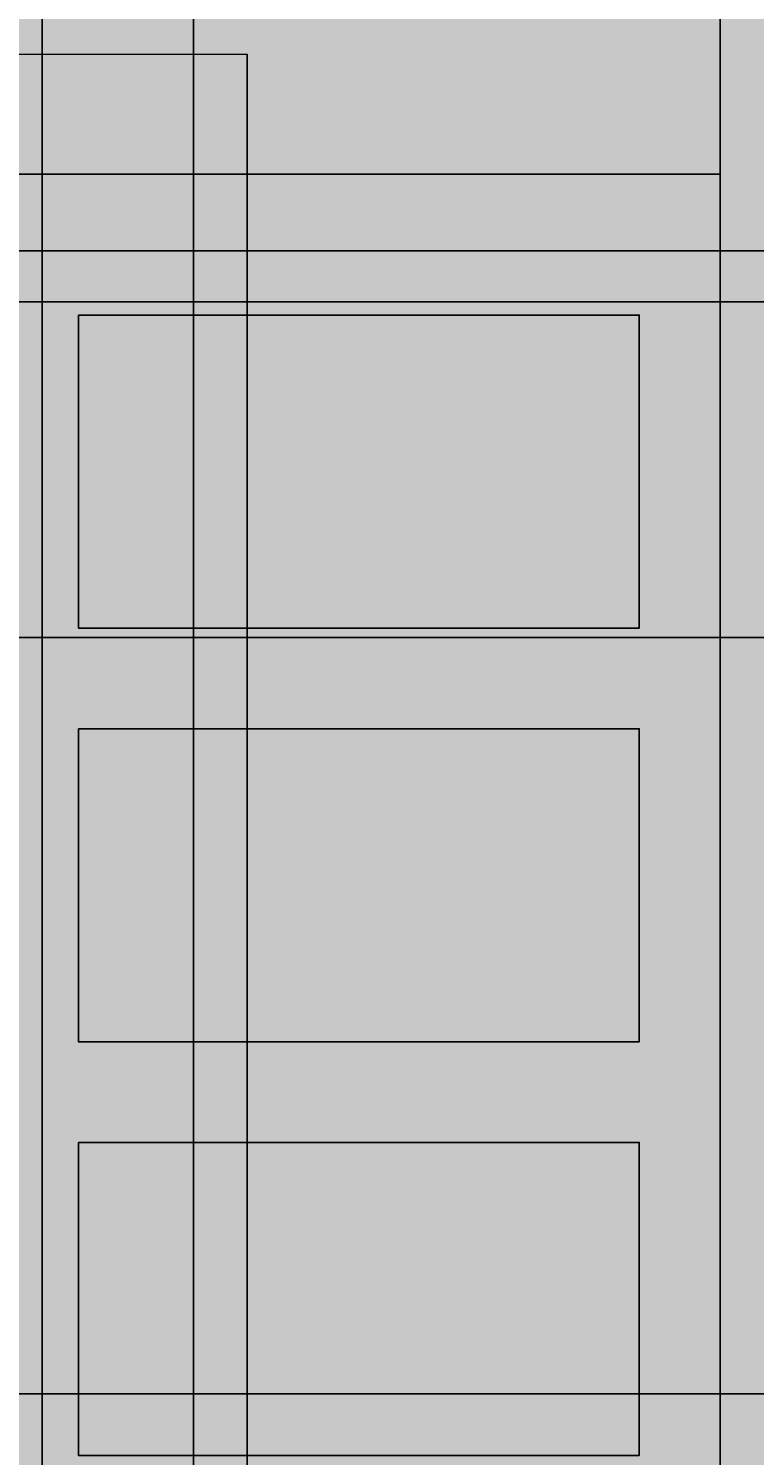
# Model space of a CAD drawing. Units: inches. Extents: x 3024 to 4744, y 1110 to 2100.
# Tile 7 of 29: x 3275 to 3332, y 1181 to 1293. Entities that reach past the tile are written whole.
import ezdxf

# ---------------------------------------------------------------- set-up
doc = ezdxf.new("R2010")
doc.units = ezdxf.units.IN
for name, color, linetype, lineweight in [('A-ANNO-DIMS', 2, 'Continuous', 18), ('A-ELEV', 7, 'Continuous', 25), ('A-ELEV-PATT', 252, 'Continuous', 13), ('A-GLAZ', 4, 'Continuous', 18)]:
    doc.layers.add(name, color=color, linetype=linetype, lineweight=lineweight)
doc.styles.get("Standard").update_dxf_attribs({"font": 'arial.ttf'})
doc.dimstyles.get("Standard").update_dxf_attribs({"dimtxt": 0.18, "dimasz": 0.18, "dimexe": 0.18, "dimexo": 0.0625, "dimgap": 0.09, "dimtad": 0, "dimtih": 1, "dimtoh": 1, "dimdec": 1, "dimzin": 0, "dimdsep": 46, "dimlunit": 3, "dimtxsty": 'Standard', "dimcen": 0.09, "dimadec": 0, "dimazin": 0, "dimtfac": 1, "dimtdec": 1, "dimtofl": 0, "dimtmove": 0, "dimatfit": 3, "dimfxl": 1, "dimtolj": 1, "dimtzin": 0, "dimarcsym": 0})

# ---------------------------------------------------------------- blocks, each defined once
blk = doc.blocks.new('WIN-BALCONY-A')
blk.add_line((3169.4, 1795.04), (3292.61, 1795.04))
blk.add_line((3169.4, 1795.04), (3292.61, 1795.04))
blk.add_lwpolyline([(3276.51, 1795.04), (3288.38, 1795.04), (3288.38, 1806.87), (3276.51, 1806.87)], close=True)
blk.add_lwpolyline([(3276.51, 1795.04), (3288.38, 1795.04), (3288.38, 1806.87), (3276.51, 1806.87)], close=True)
blk.add_lwpolyline([(3292.61, 1795.04), (3292.61, 1785.61), (3148.97, 1785.61), (3148.97, 1795.04)])
blk.add_lwpolyline([(3292.61, 1795.04), (3292.61, 1785.61), (3148.97, 1785.61), (3148.97, 1795.04)])
blk = doc.blocks.new('*D54')
at = {"layer": 'A-ANNO-DIMS', "color": 0, "lineweight": -2, "transparency": 16777216}
for p, q in [((3292.61, 1290.98), (3292.61, 1109.93)), ((3274.39, 1170.96), (3274.39, 1109.93)), ((3274.57, 1110.11), (3283.04, 1110.11)), ((3292.43, 1110.11), (3283.95, 1110.11))]:
    blk.add_line(p, q, dxfattribs=at)
at = {"layer": 'A-ANNO-DIMS', "color": 0, "transparency": 16777216}
for points in [[(3274.57, 1110.14), (3274.57, 1110.08), (3274.39, 1110.11)], [(3292.43, 1110.14), (3292.43, 1110.08), (3292.61, 1110.11)]]:
    blk.add_solid(points, dxfattribs=at)
at = {"layer": 'Defpoints', "color": 0, "transparency": 16777216}
for p in [(3292.61, 1291.04), (3274.39, 1171.02), (3292.61, 1110.11)]:
    blk.add_point(p, dxfattribs=at)
at = {"layer": 'A-ANNO-DIMS', "color": 0, "transparency": 16777216, "insert": (3283.5, 1110.11), "char_height": 0.18, "attachment_point": 5}
blk.add_mtext('\\A1;18.217', dxfattribs=at)
blk = doc.blocks.new('*D55')
at = {"layer": 'A-ANNO-DIMS', "color": 0, "lineweight": -2, "transparency": 16777216}
for p, q in [((3292.61, 1290.98), (3292.61, 1109.93)), ((3329.7, 1155.55), (3329.7, 1109.93)), ((3292.79, 1110.11), (3310.85, 1110.11)), ((3329.52, 1110.11), (3311.46, 1110.11))]:
    blk.add_line(p, q, dxfattribs=at)
at = {"layer": 'A-ANNO-DIMS', "color": 0, "transparency": 16777216}
for points in [[(3292.79, 1110.14), (3292.79, 1110.08), (3292.61, 1110.11)], [(3329.52, 1110.14), (3329.52, 1110.08), (3329.7, 1110.11)]]:
    blk.add_solid(points, dxfattribs=at)
at = {"layer": 'Defpoints', "color": 0, "transparency": 16777216}
for p in [(3292.61, 1291.04), (3329.7, 1155.61), (3329.7, 1110.11)]:
    blk.add_point(p, dxfattribs=at)
at = {"layer": 'A-ANNO-DIMS', "color": 0, "transparency": 16777216, "insert": (3311.15, 1110.11), "char_height": 0.18, "attachment_point": 5}
blk.add_mtext('\\A1;37.1', dxfattribs=at)
blk = doc.blocks.new('*D56')
at = {"layer": 'A-ANNO-DIMS', "color": 0, "lineweight": -2, "transparency": 16777216}
for p, q in [((3361.22, 1329.46), (3361.22, 1109.93)), ((3329.7, 1155.55), (3329.7, 1109.93)), ((3329.88, 1110.11), (3345.07, 1110.11)), ((3361.04, 1110.11), (3345.86, 1110.11))]:
    blk.add_line(p, q, dxfattribs=at)
at = {"layer": 'A-ANNO-DIMS', "color": 0, "transparency": 16777216}
for points in [[(3329.88, 1110.14), (3329.88, 1110.08), (3329.7, 1110.11)], [(3361.04, 1110.14), (3361.04, 1110.08), (3361.22, 1110.11)]]:
    blk.add_solid(points, dxfattribs=at)
at = {"layer": 'Defpoints', "color": 0, "transparency": 16777216}
for p in [(3361.22, 1329.52), (3329.7, 1155.61), (3361.22, 1110.11)]:
    blk.add_point(p, dxfattribs=at)
at = {"layer": 'A-ANNO-DIMS', "color": 0, "transparency": 16777216, "insert": (3345.46, 1110.11), "char_height": 0.18, "attachment_point": 5}
blk.add_mtext('\\A1;31.52', dxfattribs=at)
blk = doc.blocks.new('*D64')
at = {"layer": 'A-ANNO-DIMS', "color": 0, "lineweight": -2, "transparency": 16777216}
for p, q in [((3069.79, 1241.5), (3069.79, 2100.44)), ((3069.97, 2100.26), (3405.08, 2100.26)), ((3740.97, 2100.26), (3405.87, 2100.26)), ((3741.15, 1241.5), (3741.15, 2100.44))]:
    blk.add_line(p, q, dxfattribs=at)
at = {"layer": 'A-ANNO-DIMS', "color": 0, "transparency": 16777216}
for points in [[(3069.97, 2100.29), (3069.97, 2100.23), (3069.79, 2100.26)], [(3740.97, 2100.29), (3740.97, 2100.23), (3741.15, 2100.26)]]:
    blk.add_solid(points, dxfattribs=at)
at = {"layer": 'Defpoints', "color": 0, "transparency": 16777216}
for p in [(3741.15, 2100.26), (3069.79, 1241.43), (3741.15, 1241.43)]:
    blk.add_point(p, dxfattribs=at)
at = {"layer": 'A-ANNO-DIMS', "color": 0, "transparency": 16777216, "insert": (3405.47, 2100.26), "char_height": 0.18, "attachment_point": 5}
blk.add_mtext('\\A1;671.4', dxfattribs=at)
blk = doc.blocks.new('*D94')
at = {"layer": 'A-ANNO-DIMS', "color": 0, "lineweight": -2, "transparency": 16777216}
for p, q in [((3276.51, 1794.98), (3276.51, 1109.93)), ((3288.38, 1794.98), (3288.38, 1109.93)), ((3276.69, 1110.11), (3281.99, 1110.11)), ((3288.2, 1110.11), (3282.9, 1110.11))]:
    blk.add_line(p, q, dxfattribs=at)
at = {"layer": 'A-ANNO-DIMS', "color": 0, "transparency": 16777216}
for points in [[(3276.69, 1110.14), (3276.69, 1110.08), (3276.51, 1110.11)], [(3288.2, 1110.14), (3288.2, 1110.08), (3288.38, 1110.11)]]:
    blk.add_solid(points, dxfattribs=at)
at = {"layer": 'Defpoints', "color": 0, "transparency": 16777216}
for p in [(3276.51, 1795.04), (3288.38, 1795.04), (3288.38, 1110.11)]:
    blk.add_point(p, dxfattribs=at)
at = {"layer": 'A-ANNO-DIMS', "color": 0, "transparency": 16777216, "insert": (3282.44, 1110.11), "char_height": 0.18, "attachment_point": 5}
blk.add_mtext('\\A1;11.866', dxfattribs=at)
blk = doc.blocks.new('*D120')
at = {"layer": 'A-ANNO-DIMS', "color": 0, "lineweight": -2, "transparency": 16777216}
for p, q in [((3270.45, 1271.61), (3786.83, 1271.61)), ((3786.65, 1271.43), (3786.65, 1221.5)), ((3786.65, 1171.2), (3786.65, 1221.14)), ((3274.45, 1171.02), (3786.83, 1171.02))]:
    blk.add_line(p, q, dxfattribs=at)
at = {"layer": 'A-ANNO-DIMS', "color": 0, "transparency": 16777216}
for points in [[(3786.62, 1271.43), (3786.68, 1271.43), (3786.65, 1271.61)], [(3786.62, 1171.2), (3786.68, 1171.2), (3786.65, 1171.02)]]:
    blk.add_solid(points, dxfattribs=at)
at = {"layer": 'Defpoints', "color": 0, "transparency": 16777216}
for p in [(3270.39, 1271.61), (3786.65, 1271.61), (3274.39, 1171.02)]:
    blk.add_point(p, dxfattribs=at)
at = {"layer": 'A-ANNO-DIMS', "color": 0, "transparency": 16777216, "insert": (3786.65, 1221.32), "char_height": 0.18, "attachment_point": 5}
blk.add_mtext('\\A1;100.59', dxfattribs=at)
blk = doc.blocks.new('*D121')
at = {"layer": 'A-ANNO-DIMS', "color": 0, "lineweight": -2, "transparency": 16777216}
for p, q in [((3274.45, 1275.61), (3786.83, 1275.61)), ((3786.65, 1275.43), (3786.65, 1273.79)), ((3786.65, 1271.79), (3786.65, 1273.43)), ((3270.45, 1271.61), (3786.83, 1271.61))]:
    blk.add_line(p, q, dxfattribs=at)
at = {"layer": 'A-ANNO-DIMS', "color": 0, "transparency": 16777216}
for points in [[(3786.62, 1275.43), (3786.68, 1275.43), (3786.65, 1275.61)], [(3786.62, 1271.79), (3786.68, 1271.79), (3786.65, 1271.61)]]:
    blk.add_solid(points, dxfattribs=at)
at = {"layer": 'Defpoints', "color": 0, "transparency": 16777216}
for p in [(3274.39, 1275.61), (3786.65, 1275.61), (3270.39, 1271.61)]:
    blk.add_point(p, dxfattribs=at)
at = {"layer": 'A-ANNO-DIMS', "color": 0, "transparency": 16777216, "insert": (3786.65, 1273.61), "char_height": 0.18, "attachment_point": 5}
blk.add_mtext('\\A1;4.00', dxfattribs=at)
blk = doc.blocks.new('*D122')
at = {"layer": 'A-ANNO-DIMS', "color": 0, "lineweight": -2, "transparency": 16777216}
for p, q in [((3228.45, 1185.95), (3786.83, 1185.95)), ((3786.65, 1185.77), (3786.65, 1178.67)), ((3786.65, 1171.2), (3786.65, 1178.31)), ((3270.45, 1171.02), (3786.83, 1171.02))]:
    blk.add_line(p, q, dxfattribs=at)
at = {"layer": 'A-ANNO-DIMS', "color": 0, "transparency": 16777216}
for points in [[(3786.62, 1185.77), (3786.68, 1185.77), (3786.65, 1185.95)], [(3786.62, 1171.2), (3786.68, 1171.2), (3786.65, 1171.02)]]:
    blk.add_solid(points, dxfattribs=at)
at = {"layer": 'Defpoints', "color": 0, "transparency": 16777216}
for p in [(3228.39, 1185.95), (3270.39, 1171.02), (3786.65, 1171.02)]:
    blk.add_point(p, dxfattribs=at)
at = {"layer": 'A-ANNO-DIMS', "color": 0, "transparency": 16777216, "insert": (3786.65, 1178.49), "char_height": 0.18, "attachment_point": 5}
blk.add_mtext('\\A1;14.928', dxfattribs=at)
blk = doc.blocks.new('*D123')
at = {"layer": 'A-ANNO-DIMS', "color": 0, "lineweight": -2, "transparency": 16777216}
for p, q in [((3228.45, 1245.27), (3786.83, 1245.27)), ((3786.65, 1245.09), (3786.65, 1215.79)), ((3786.65, 1186.13), (3786.65, 1215.43)), ((3228.45, 1185.95), (3786.83, 1185.95))]:
    blk.add_line(p, q, dxfattribs=at)
at = {"layer": 'A-ANNO-DIMS', "color": 0, "transparency": 16777216}
for points in [[(3786.62, 1245.09), (3786.68, 1245.09), (3786.65, 1245.27)], [(3786.62, 1186.13), (3786.68, 1186.13), (3786.65, 1185.95)]]:
    blk.add_solid(points, dxfattribs=at)
at = {"layer": 'Defpoints', "color": 0, "transparency": 16777216}
for p in [(3228.39, 1245.27), (3786.65, 1245.27), (3228.39, 1185.95)]:
    blk.add_point(p, dxfattribs=at)
at = {"layer": 'A-ANNO-DIMS', "color": 0, "transparency": 16777216, "insert": (3786.65, 1215.61), "char_height": 0.18, "attachment_point": 5}
blk.add_mtext('\\A1;59.32', dxfattribs=at)

msp = doc.modelspace()

# ---------------------------------------------------------------- hatches: boundary and pattern name
at = {"layer": 'A-ELEV-PATT'}
h = msp.add_hatch(color=256, dxfattribs=at)
h.dxf.hatch_style = 1
h.paths.add_polyline_path([(3491.8271, 2054.7584), (3320.5658, 2054.7584), (3320.5658, 2043.5286), (3491.8271, 2043.5286)])
h.paths.add_polyline_path([(3292.6051, 1905.6112), (3148.9694, 1905.6112), (3148.9694, 1897.4879), (3169.3964, 1897.4879), (3292.6051, 1897.4879)])
h.paths.add_polyline_path([(3292.6051, 1795.0431), (3169.3964, 1795.0431), (3148.9694, 1795.0431), (3148.9694, 1785.6112), (3292.6051, 1785.6112)])
h.paths.add_polyline_path([(3292.6051, 1779.6112), (3148.9694, 1779.6112), (3148.9694, 1771.4879), (3169.3964, 1771.4879), (3292.6051, 1771.4879)])
h.paths.add_polyline_path([(3292.6051, 1669.0431), (3169.3964, 1669.0431), (3148.9694, 1669.0431), (3148.9694, 1659.6112), (3292.6051, 1659.6112)])
h.paths.add_polyline_path([(3292.6051, 1653.6112), (3148.9694, 1653.6112), (3148.9694, 1645.4879), (3169.3964, 1645.4879), (3292.6051, 1645.4879)])
h.paths.add_polyline_path([(3292.6051, 1543.0431), (3169.3964, 1543.0431), (3148.9694, 1543.0431), (3148.9694, 1533.6112), (3292.6051, 1533.6112)])
h.paths.add_polyline_path([(3292.6051, 1527.6112), (3148.9694, 1527.6112), (3148.9694, 1519.4879), (3169.3964, 1519.4879), (3292.6051, 1519.4879)])
h.paths.add_polyline_path([(3292.6051, 1401.6112), (3148.9694, 1401.6112), (3148.9694, 1393.4879), (3169.3964, 1393.4879), (3292.6051, 1393.4879)])
h.paths.add_polyline_path([(3292.6051, 1417.0431), (3169.3964, 1417.0431), (3148.9694, 1417.0431), (3148.9694, 1407.6112), (3292.6051, 1407.6112)])
h.paths.add_polyline_path([(3292.6051, 1291.0431), (3169.3964, 1291.0431), (3148.9694, 1291.0431), (3148.9694, 1281.6112), (3292.6051, 1281.6112)])
h.paths.add_polyline_path([(3654.037, 1165.0431), (3530.8283, 1165.0431), (3510.4013, 1165.0431), (3510.4013, 1155.6112), (3654.037, 1155.6112)])
h.paths.add_polyline_path([(3654.037, 1275.6112), (3510.4013, 1275.6112), (3510.4013, 1267.4879), (3530.8283, 1267.4879), (3654.037, 1267.4879)])
h.paths.add_polyline_path([(3654.037, 1291.0431), (3530.8283, 1291.0431), (3510.4013, 1291.0431), (3510.4013, 1281.6112), (3654.037, 1281.6112)])
h.paths.add_polyline_path([(3654.037, 1417.0431), (3530.8283, 1417.0431), (3510.4013, 1417.0431), (3510.4013, 1407.6112), (3654.037, 1407.6112)])
h.paths.add_polyline_path([(3654.037, 1401.6112), (3510.4013, 1401.6112), (3510.4013, 1393.4879), (3530.8283, 1393.4879), (3654.037, 1393.4879)])
h.paths.add_polyline_path([(3654.037, 1543.0431), (3530.8283, 1543.0431), (3510.4013, 1543.0431), (3510.4013, 1533.6112), (3654.037, 1533.6112)])
h.paths.add_polyline_path([(3654.037, 1527.6112), (3510.4013, 1527.6112), (3510.4013, 1519.4879), (3530.8283, 1519.4879), (3654.037, 1519.4879)])
h.paths.add_polyline_path([(3654.037, 1653.6112), (3510.4013, 1653.6112), (3510.4013, 1645.4879), (3530.8283, 1645.4879), (3654.037, 1645.4879)])
h.paths.add_polyline_path([(3654.037, 1669.0431), (3530.8283, 1669.0431), (3510.4013, 1669.0431), (3510.4013, 1659.6112), (3654.037, 1659.6112)])
h.paths.add_polyline_path([(3654.037, 1779.6112), (3510.4013, 1779.6112), (3510.4013, 1771.4879), (3530.8283, 1771.4879), (3654.037, 1771.4879)])
h.paths.add_polyline_path([(3654.037, 1795.0431), (3530.8283, 1795.0431), (3510.4013, 1795.0431), (3510.4013, 1785.6112), (3654.037, 1785.6112)])
h.paths.add_polyline_path([(3654.037, 1905.6112), (3510.4013, 1905.6112), (3510.4013, 1897.4879), (3530.8283, 1897.4879), (3654.037, 1897.4879)])
h = msp.add_hatch(color=256, dxfattribs=at)
h.dxf.hatch_style = 1
h.paths.add_polyline_path([(3335.1044, 2043.5286), (3329.7033, 2043.5286), (3329.7033, 1155.6112), (3335.1044, 1155.6112)])
h.paths.add_polyline_path([(3481.2411, 2043.5286), (3335.1044, 2043.5286), (3335.1044, 1155.6112), (3481.2411, 1155.6112)])
h.paths.add_polyline_path([(3449.7202, 1329.5246), (3361.2242, 1329.5246), (3361.2242, 1436.6064), (3449.7202, 1436.6064)], flags=16)
h.paths.add_polyline_path([(3445.7202, 1333.5246), (3365.2242, 1333.5246), (3365.2242, 1432.6064), (3445.7202, 1432.6064)], flags=0)
h.paths.add_polyline_path([(3449.7202, 1455.5246), (3361.2242, 1455.5246), (3361.2242, 1562.6064), (3449.7202, 1562.6064)], flags=16)
h.paths.add_polyline_path([(3445.7202, 1459.5246), (3365.2242, 1459.5246), (3365.2242, 1558.6064), (3445.7202, 1558.6064)], flags=0)
h.paths.add_polyline_path([(3449.7202, 1581.5246), (3361.2242, 1581.5246), (3361.2242, 1688.6064), (3449.7202, 1688.6064)], flags=16)
h.paths.add_polyline_path([(3445.7202, 1585.5246), (3365.2242, 1585.5246), (3365.2242, 1684.6064), (3445.7202, 1684.6064)], flags=0)
h.paths.add_polyline_path([(3449.7202, 1707.5246), (3361.2242, 1707.5246), (3361.2242, 1814.6064), (3449.7202, 1814.6064)], flags=16)
h.paths.add_polyline_path([(3445.7202, 1711.5246), (3365.2242, 1711.5246), (3365.2242, 1810.6064), (3445.7202, 1810.6064)], flags=0)
h.paths.add_polyline_path([(3449.7202, 1833.5246), (3361.2242, 1833.5246), (3361.2242, 1940.6064), (3449.7202, 1940.6064)], flags=16)
h.paths.add_polyline_path([(3445.7202, 1837.5246), (3365.2242, 1837.5246), (3365.2242, 1936.6064), (3445.7202, 1936.6064)], flags=0)
h = msp.add_hatch(color=256, dxfattribs=at)
h.dxf.hatch_style = 1
h.paths.add_polyline_path([(3329.7033, 1407.6112), (3105.4722, 1407.6112), (3105.4722, 1401.6112), (3329.7033, 1401.6112)])
h.paths.add_polyline_path([(3329.7033, 1281.6112), (3105.4722, 1281.6112), (3105.4722, 1275.6112), (3112.3838, 1275.6112), (3329.7033, 1275.6112)])
h.paths.add_polyline_path([(3329.7033, 1533.6112), (3105.4722, 1533.6112), (3105.4722, 1527.6112), (3329.7033, 1527.6112)])
h.paths.add_polyline_path([(3329.7033, 1659.6112), (3105.4722, 1659.6112), (3105.4722, 1653.6112), (3329.7033, 1653.6112)])
h.paths.add_polyline_path([(3329.7033, 1785.6112), (3105.4722, 1785.6112), (3105.4722, 1779.6112), (3329.7033, 1779.6112)])
h.paths.add_polyline_path([(3329.7033, 1911.6112), (3105.4722, 1911.6112), (3095.7158, 1911.6112), (3095.7158, 1905.6112), (3329.7033, 1905.6112)])
h.paths.add_polyline_path([(3715.2286, 1911.6112), (3705.4722, 1911.6112), (3705.4722, 1905.6112), (3715.2286, 1905.6112)])
h.paths.add_polyline_path([(3688.5588, 1911.6112), (3481.2411, 1911.6112), (3481.2411, 1905.6112), (3688.5588, 1905.6112)])
h = msp.add_hatch(color=256, dxfattribs=at)
h.dxf.hatch_style = 1
h.paths.add_polyline_path([(3154.3287, 1897.4879), (3148.9694, 1897.4879), (3148.9694, 1905.6112), (3105.4722, 1905.6112), (3105.4722, 1785.6112), (3148.9694, 1785.6112), (3148.9694, 1795.0431), (3151.6604, 1795.0431), (3151.6604, 1806.8674), (3154.3287, 1806.8674)])
h.paths.add_polyline_path([(3329.7033, 1905.6112), (3292.6051, 1905.6112), (3292.6051, 1897.4879), (3287.2458, 1897.4879), (3287.2458, 1806.8674), (3288.3759, 1806.8674), (3288.3759, 1795.0431), (3292.6051, 1795.0431), (3292.6051, 1785.6112), (3329.7033, 1785.6112)])
h.paths.add_polyline_path([(3154.3287, 1771.4879), (3148.9694, 1771.4879), (3148.9694, 1779.6112), (3105.4722, 1779.6112), (3105.4722, 1659.6112), (3148.9694, 1659.6112), (3148.9694, 1669.0431), (3151.6604, 1669.0431), (3151.6604, 1680.8674), (3154.3287, 1680.8674)])
h.paths.add_polyline_path([(3329.7033, 1779.6112), (3292.6051, 1779.6112), (3292.6051, 1771.4879), (3287.2458, 1771.4879), (3287.2458, 1680.8674), (3288.3759, 1680.8674), (3288.3759, 1669.0431), (3292.6051, 1669.0431), (3292.6051, 1659.6112), (3329.7033, 1659.6112)])
h.paths.add_polyline_path([(3154.3287, 1645.4879), (3148.9694, 1645.4879), (3148.9694, 1653.6112), (3105.4722, 1653.6112), (3105.4722, 1533.6112), (3148.9694, 1533.6112), (3148.9694, 1543.0431), (3151.6604, 1543.0431), (3151.6604, 1554.8674), (3154.3287, 1554.8674)])
h.paths.add_polyline_path([(3329.7033, 1653.6112), (3292.6051, 1653.6112), (3292.6051, 1645.4879), (3287.2458, 1645.4879), (3287.2458, 1554.8674), (3288.3759, 1554.8674), (3288.3759, 1543.0431), (3292.6051, 1543.0431), (3292.6051, 1533.6112), (3329.7033, 1533.6112)])
h.paths.add_polyline_path([(3329.7033, 1527.6112), (3292.6051, 1527.6112), (3292.6051, 1519.4879), (3287.2458, 1519.4879), (3287.2458, 1428.8674), (3288.3759, 1428.8674), (3288.3759, 1417.0431), (3292.6051, 1417.0431), (3292.6051, 1407.6112), (3329.7033, 1407.6112)])
h.paths.add_polyline_path([(3329.7033, 1401.6112), (3292.6051, 1401.6112), (3292.6051, 1393.4879), (3287.2458, 1393.4879), (3287.2458, 1302.8674), (3288.3759, 1302.8674), (3288.3759, 1291.0431), (3292.6051, 1291.0431), (3292.6051, 1281.6112), (3329.7033, 1281.6112)])
h.paths.add_polyline_path([(3154.3287, 1393.4879), (3148.9694, 1393.4879), (3148.9694, 1401.6112), (3105.4722, 1401.6112), (3105.4722, 1281.6112), (3148.9694, 1281.6112), (3148.9694, 1291.0431), (3151.6604, 1291.0431), (3151.6604, 1302.8674), (3154.3287, 1302.8674)])
h.paths.add_polyline_path([(3154.3287, 1519.4879), (3148.9694, 1519.4879), (3148.9694, 1527.6112), (3105.4722, 1527.6112), (3105.4722, 1407.6112), (3148.9694, 1407.6112), (3148.9694, 1417.0431), (3151.6604, 1417.0431), (3151.6604, 1428.8674), (3154.3287, 1428.8674)])
h.paths.add_polyline_path([(3515.7606, 1897.4879), (3510.4013, 1897.4879), (3510.4013, 1905.6112), (3481.2411, 1905.6112), (3481.2411, 1785.6112), (3510.4013, 1785.6112), (3510.4013, 1795.0431), (3513.0923, 1795.0431), (3513.0923, 1806.8674), (3515.7606, 1806.8674)])
h.paths.add_polyline_path([(3688.5588, 1905.6112), (3654.037, 1905.6112), (3654.037, 1897.4879), (3648.6777, 1897.4879), (3648.6777, 1806.8674), (3649.8078, 1806.8674), (3649.8078, 1795.0431), (3654.037, 1795.0431), (3654.037, 1785.6112), (3688.5588, 1785.6112)])
h.paths.add_polyline_path([(3515.7606, 1771.4879), (3510.4013, 1771.4879), (3510.4013, 1779.6112), (3481.2411, 1779.6112), (3481.2411, 1659.6112), (3510.4013, 1659.6112), (3510.4013, 1669.0431), (3513.0923, 1669.0431), (3513.0923, 1680.8674), (3515.7606, 1680.8674)])
h.paths.add_polyline_path([(3688.5588, 1779.6112), (3654.037, 1779.6112), (3654.037, 1771.4879), (3648.6777, 1771.4879), (3648.6777, 1680.8674), (3649.8078, 1680.8674), (3649.8078, 1669.0431), (3654.037, 1669.0431), (3654.037, 1659.6112), (3688.5588, 1659.6112)])
h.paths.add_polyline_path([(3515.7606, 1645.4879), (3510.4013, 1645.4879), (3510.4013, 1653.6112), (3481.2411, 1653.6112), (3481.2411, 1533.6112), (3510.4013, 1533.6112), (3510.4013, 1543.0431), (3513.0923, 1543.0431), (3513.0923, 1554.8674), (3515.7606, 1554.8674)])
h.paths.add_polyline_path([(3688.5588, 1653.6112), (3654.037, 1653.6112), (3654.037, 1645.4879), (3648.6777, 1645.4879), (3648.6777, 1554.8674), (3649.8078, 1554.8674), (3649.8078, 1543.0431), (3654.037, 1543.0431), (3654.037, 1533.6112), (3688.5588, 1533.6112)])
h.paths.add_polyline_path([(3515.7606, 1519.4879), (3510.4013, 1519.4879), (3510.4013, 1527.6112), (3481.2411, 1527.6112), (3481.2411, 1407.6112), (3510.4013, 1407.6112), (3510.4013, 1417.0431), (3513.0923, 1417.0431), (3513.0923, 1428.8674), (3515.7606, 1428.8674)])
h.paths.add_polyline_path([(3688.5588, 1527.6112), (3654.037, 1527.6112), (3654.037, 1519.4879), (3648.6777, 1519.4879), (3648.6777, 1428.8674), (3649.8078, 1428.8674), (3649.8078, 1417.0431), (3654.037, 1417.0431), (3654.037, 1407.6112), (3688.5588, 1407.6112)])
h.paths.add_polyline_path([(3515.7606, 1393.4879), (3510.4013, 1393.4879), (3510.4013, 1401.6112), (3481.2411, 1401.6112), (3481.2411, 1281.6112), (3510.4013, 1281.6112), (3510.4013, 1291.0431), (3513.0923, 1291.0431), (3513.0923, 1302.8674), (3515.7606, 1302.8674)])
h.paths.add_polyline_path([(3688.5588, 1401.6112), (3654.037, 1401.6112), (3654.037, 1393.4879), (3648.6777, 1393.4879), (3648.6777, 1302.8674), (3649.8078, 1302.8674), (3649.8078, 1291.0431), (3654.037, 1291.0431), (3654.037, 1281.6112), (3688.5588, 1281.6112)])
h.paths.add_polyline_path([(3515.7606, 1267.4879), (3510.4013, 1267.4879), (3510.4013, 1275.6112), (3481.2411, 1275.6112), (3481.2411, 1155.6112), (3510.4013, 1155.6112), (3510.4013, 1165.0431), (3513.0923, 1165.0431), (3513.0923, 1176.8674), (3515.7606, 1176.8674)])
h.paths.add_polyline_path([(3688.5588, 1275.6112), (3654.037, 1275.6112), (3654.037, 1267.4879), (3648.6777, 1267.4879), (3648.6777, 1176.8674), (3649.8078, 1176.8674), (3649.8078, 1165.0431), (3654.037, 1165.0431), (3654.037, 1155.6112), (3688.5588, 1155.6112)])
h.paths.add_polyline_path([(3112.3838, 1275.6112), (3105.4722, 1275.6112), (3105.4722, 1171.0239), (3112.3838, 1171.0239)])
h = msp.add_hatch(color=256, dxfattribs=at)
h.dxf.hatch_style = 1
h.paths.add_polyline_path([(3169.3964, 1897.4879), (3160.8586, 1897.4879), (3160.8586, 1806.8674), (3163.5269, 1806.8674), (3163.5269, 1795.0431), (3169.3964, 1795.0431)])
h.paths.add_polyline_path([(3280.716, 1897.4879), (3272.1781, 1897.4879), (3272.1781, 1795.0431), (3276.5094, 1795.0431), (3276.5094, 1806.8674), (3280.716, 1806.8674)])
h.paths.add_polyline_path([(3280.716, 1771.4879), (3272.1781, 1771.4879), (3272.1781, 1669.0431), (3276.5094, 1669.0431), (3276.5094, 1680.8674), (3280.716, 1680.8674)])
h.paths.add_polyline_path([(3169.3964, 1771.4879), (3160.8586, 1771.4879), (3160.8586, 1680.8674), (3163.5269, 1680.8674), (3163.5269, 1669.0431), (3169.3964, 1669.0431)])
h.paths.add_polyline_path([(3169.3964, 1645.4879), (3160.8586, 1645.4879), (3160.8586, 1554.8674), (3163.5269, 1554.8674), (3163.5269, 1543.0431), (3169.3964, 1543.0431)])
h.paths.add_polyline_path([(3280.716, 1645.4879), (3272.1781, 1645.4879), (3272.1781, 1543.0431), (3276.5094, 1543.0431), (3276.5094, 1554.8674), (3280.716, 1554.8674)])
h.paths.add_polyline_path([(3169.3964, 1519.4879), (3160.8586, 1519.4879), (3160.8586, 1428.8674), (3163.5269, 1428.8674), (3163.5269, 1417.0431), (3169.3964, 1417.0431)])
h.paths.add_polyline_path([(3280.716, 1519.4879), (3272.1781, 1519.4879), (3272.1781, 1417.0431), (3276.5094, 1417.0431), (3276.5094, 1428.8674), (3280.716, 1428.8674)])
h.paths.add_polyline_path([(3169.3964, 1393.4879), (3160.8586, 1393.4879), (3160.8586, 1302.8674), (3163.5269, 1302.8674), (3163.5269, 1291.0431), (3169.3964, 1291.0431)])
h.paths.add_polyline_path([(3280.716, 1393.4879), (3272.1781, 1393.4879), (3272.1781, 1291.0431), (3276.5094, 1291.0431), (3276.5094, 1302.8674), (3280.716, 1302.8674)])
h.paths.add_polyline_path([(3642.1479, 1267.4879), (3633.61, 1267.4879), (3633.61, 1165.0431), (3637.9413, 1165.0431), (3637.9413, 1176.8674), (3642.1479, 1176.8674)])
h.paths.add_polyline_path([(3530.8283, 1267.4879), (3522.2905, 1267.4879), (3522.2905, 1176.8674), (3524.9588, 1176.8674), (3524.9588, 1165.0431), (3530.8283, 1165.0431)])
h.paths.add_polyline_path([(3642.1479, 1393.4879), (3633.61, 1393.4879), (3633.61, 1291.0431), (3637.9413, 1291.0431), (3637.9413, 1302.8674), (3642.1479, 1302.8674)])
h.paths.add_polyline_path([(3530.8283, 1393.4879), (3522.2905, 1393.4879), (3522.2905, 1302.8674), (3524.9588, 1302.8674), (3524.9588, 1291.0431), (3530.8283, 1291.0431)])
h.paths.add_polyline_path([(3530.8283, 1519.4879), (3522.2905, 1519.4879), (3522.2905, 1428.8674), (3524.9588, 1428.8674), (3524.9588, 1417.0431), (3530.8283, 1417.0431)])
h.paths.add_polyline_path([(3642.1479, 1519.4879), (3633.61, 1519.4879), (3633.61, 1417.0431), (3637.9413, 1417.0431), (3637.9413, 1428.8674), (3642.1479, 1428.8674)])
h.paths.add_polyline_path([(3530.8283, 1645.4879), (3522.2905, 1645.4879), (3522.2905, 1554.8674), (3524.9588, 1554.8674), (3524.9588, 1543.0431), (3530.8283, 1543.0431)])
h.paths.add_polyline_path([(3642.1479, 1645.4879), (3633.61, 1645.4879), (3633.61, 1543.0431), (3637.9413, 1543.0431), (3637.9413, 1554.8674), (3642.1479, 1554.8674)])
h.paths.add_polyline_path([(3642.1479, 1771.4879), (3633.61, 1771.4879), (3633.61, 1669.0431), (3637.9413, 1669.0431), (3637.9413, 1680.8674), (3642.1479, 1680.8674)])
h.paths.add_polyline_path([(3530.8283, 1771.4879), (3522.2905, 1771.4879), (3522.2905, 1680.8674), (3524.9588, 1680.8674), (3524.9588, 1669.0431), (3530.8283, 1669.0431)])
h.paths.add_polyline_path([(3530.8283, 1897.4879), (3522.2905, 1897.4879), (3522.2905, 1806.8674), (3524.9588, 1806.8674), (3524.9588, 1795.0431), (3530.8283, 1795.0431)])
h.paths.add_polyline_path([(3642.1479, 1897.4879), (3633.61, 1897.4879), (3633.61, 1795.0431), (3637.9413, 1795.0431), (3637.9413, 1806.8674), (3642.1479, 1806.8674)])
h = msp.add_hatch(color=256, dxfattribs=at)
h.dxf.hatch_style = 1
h.paths.add_polyline_path([(3163.5269, 1302.8674), (3151.6604, 1302.8674), (3151.6604, 1291.0431), (3163.5269, 1291.0431)])
h.paths.add_polyline_path([(3288.3759, 1302.8674), (3276.5094, 1302.8674), (3276.5094, 1291.0431), (3288.3759, 1291.0431)])
h.paths.add_polyline_path([(3288.3759, 1428.8674), (3276.5094, 1428.8674), (3276.5094, 1417.0431), (3288.3759, 1417.0431)])
h.paths.add_polyline_path([(3163.5269, 1428.8674), (3151.6604, 1428.8674), (3151.6604, 1417.0431), (3163.5269, 1417.0431)])
h.paths.add_polyline_path([(3163.5269, 1554.8674), (3151.6604, 1554.8674), (3151.6604, 1543.0431), (3163.5269, 1543.0431)])
h.paths.add_polyline_path([(3288.3759, 1554.8674), (3276.5094, 1554.8674), (3276.5094, 1543.0431), (3288.3759, 1543.0431)])
h.paths.add_polyline_path([(3163.5269, 1680.8674), (3151.6604, 1680.8674), (3151.6604, 1669.0431), (3163.5269, 1669.0431)])
h.paths.add_polyline_path([(3288.3759, 1680.8674), (3276.5094, 1680.8674), (3276.5094, 1669.0431), (3288.3759, 1669.0431)])
h.paths.add_polyline_path([(3163.5269, 1806.8674), (3151.6604, 1806.8674), (3151.6604, 1795.0431), (3163.5269, 1795.0431)])
h.paths.add_polyline_path([(3288.3759, 1806.8674), (3276.5094, 1806.8674), (3276.5094, 1795.0431), (3288.3759, 1795.0431)])
h.paths.add_polyline_path([(3524.9588, 1806.8674), (3513.0923, 1806.8674), (3513.0923, 1795.0431), (3524.9588, 1795.0431)])
h.paths.add_polyline_path([(3649.8078, 1806.8674), (3637.9413, 1806.8674), (3637.9413, 1795.0431), (3649.8078, 1795.0431)])
h.paths.add_polyline_path([(3524.9588, 1680.8674), (3513.0923, 1680.8674), (3513.0923, 1669.0431), (3524.9588, 1669.0431)])
h.paths.add_polyline_path([(3649.8078, 1680.8674), (3637.9413, 1680.8674), (3637.9413, 1669.0431), (3649.8078, 1669.0431)])
h.paths.add_polyline_path([(3524.9588, 1554.8674), (3513.0923, 1554.8674), (3513.0923, 1543.0431), (3524.9588, 1543.0431)])
h.paths.add_polyline_path([(3649.8078, 1554.8674), (3637.9413, 1554.8674), (3637.9413, 1543.0431), (3649.8078, 1543.0431)])
h.paths.add_polyline_path([(3524.9588, 1428.8674), (3513.0923, 1428.8674), (3513.0923, 1417.0431), (3524.9588, 1417.0431)])
h.paths.add_polyline_path([(3649.8078, 1428.8674), (3637.9413, 1428.8674), (3637.9413, 1417.0431), (3649.8078, 1417.0431)])
h.paths.add_polyline_path([(3524.9588, 1302.8674), (3513.0923, 1302.8674), (3513.0923, 1291.0431), (3524.9588, 1291.0431)])
h.paths.add_polyline_path([(3649.8078, 1302.8674), (3637.9413, 1302.8674), (3637.9413, 1291.0431), (3649.8078, 1291.0431)])
h.paths.add_polyline_path([(3524.9588, 1176.8674), (3513.0923, 1176.8674), (3513.0923, 1165.0431), (3524.9588, 1165.0431)])
h.paths.add_polyline_path([(3649.8078, 1176.8674), (3637.9413, 1176.8674), (3637.9413, 1165.0431), (3649.8078, 1165.0431)])
h = msp.add_hatch(color=256, dxfattribs=at)
h.dxf.hatch_style = 1
h.paths.add_polyline_path([(3329.7033, 1275.6112), (3274.3877, 1275.6112), (3274.3877, 1171.0239), (3329.7033, 1171.0239)])
h.paths.add_polyline_path([(3323.3693, 1246.0161), (3279.3584, 1246.0161), (3279.3584, 1270.5642), (3323.3693, 1270.5642)], flags=16)
h.paths.add_polyline_path([(3323.3693, 1238.118), (3323.3693, 1213.5699), (3279.3584, 1213.5699), (3279.3584, 1238.118)], flags=16)
h.paths.add_polyline_path([(3323.3693, 1205.6718), (3323.3693, 1181.1236), (3279.3584, 1181.1236), (3279.3584, 1205.6718)], flags=16)
h.paths.add_polyline_path([(3170.1608, 1275.6112), (3112.3838, 1275.6112), (3112.3838, 1171.0239), (3118.1176, 1171.0239), (3170.1608, 1171.0239)])
h.paths.add_polyline_path([(3120.3696, 1246.0161), (3120.3696, 1270.5642), (3164.3806, 1270.5642), (3164.3806, 1246.0161)], flags=16)
h.paths.add_polyline_path([(3120.3696, 1238.118), (3164.3806, 1238.118), (3164.3806, 1213.5699), (3120.3696, 1213.5699)], flags=16)
h.paths.add_polyline_path([(3120.3696, 1205.6718), (3164.3806, 1205.6718), (3164.3806, 1181.1236), (3120.3696, 1181.1236)], flags=16)
h = msp.add_hatch(color=256, dxfattribs=at)
h.dxf.hatch_style = 1
h.paths.add_polyline_path([(3323.3693, 1270.5642), (3279.3584, 1270.5642), (3279.3584, 1246.0161), (3323.3693, 1246.0161)])
h.paths.add_polyline_path([(3323.3693, 1238.118), (3279.3584, 1238.118), (3279.3584, 1213.5699), (3323.3693, 1213.5699)])
h.paths.add_polyline_path([(3323.3693, 1205.6718), (3279.3584, 1205.6718), (3279.3584, 1181.1236), (3323.3693, 1181.1236)])
h.paths.add_polyline_path([(3164.3806, 1270.5642), (3120.3696, 1270.5642), (3120.3696, 1246.0161), (3164.3806, 1246.0161)])
h.paths.add_polyline_path([(3164.3806, 1238.118), (3120.3696, 1238.118), (3120.3696, 1213.5699), (3164.3806, 1213.5699)])
h.paths.add_polyline_path([(3164.3806, 1205.6718), (3120.3696, 1205.6718), (3120.3696, 1181.1236), (3164.3806, 1181.1236)])

# ---------------------------------------------------------------- linework, layer by layer
at = {"layer": 'A-ELEV'}
for p, q in [((3105.4722, 1281.6112), (3329.7033, 1281.6112)), ((3105.4722, 1281.6112), (3329.7033, 1281.6112)), ((3329.7033, 1275.6112), (3105.4722, 1275.6112)), ((3329.7033, 1275.6112), (3105.4722, 1275.6112))]:
    msp.add_line(p, q, dxfattribs=at)
for points in [[(3481.2411, 1155.6112), (3329.7033, 1155.6112), (3329.7033, 2043.5286), (3481.2411, 2043.5286)], [(3329.7033, 2043.5286), (3335.1044, 2043.5286), (3335.1044, 1155.6112), (3329.7033, 1155.6112)], [(3481.2411, 1155.6112), (3329.7033, 1155.6112), (3329.7033, 2043.5286), (3481.2411, 2043.5286)], [(3329.7033, 2043.5286), (3335.1044, 2043.5286), (3335.1044, 1155.6112), (3329.7033, 1155.6112)], [(3279.3584, 1270.5642), (3323.3693, 1270.5642), (3323.3693, 1246.0161), (3279.3584, 1246.0161)], [(3279.3584, 1238.118), (3323.3693, 1238.118), (3323.3693, 1213.5699), (3279.3584, 1213.5699)], [(3279.3584, 1205.6718), (3323.3693, 1205.6718), (3323.3693, 1181.1236), (3279.3584, 1181.1236)]]:
    msp.add_lwpolyline(points, close=True, dxfattribs=at)

# ---------------------------------------------------------------- block references
at = {"layer": 'A-GLAZ'}
msp.add_blockref('WIN-BALCONY-A', (0, -504), dxfattribs=at)

# ---------------------------------------------------------------- dimensions: what is measured, and where the dimension line sits
at = {"layer": 'A-ANNO-DIMS'}
for base, p1, p2, override, picture, middle in [((3741.1507, 2100.2584), (3069.7937, 1241.4341), (3741.1507, 1241.4341), {"dimdec": 1, "dimlfac": 1, "dimrnd": 0, "dimzin": 0, "dimdsep": 46, "dimlunit": 2}, '*D64', (3405.4722, 2100.2584)), ((3288.37586, 1110.111173), (3276.509363, 1795.043127), (3288.37586, 1795.043127), {"dimdec": 3, "dimlfac": 1, "dimrnd": 0, "dimzin": 0, "dimdsep": 46, "dimlunit": 2}, '*D94', (3282.442612, 1110.111173)), ((3361.2242, 1110.1112), (3329.7033, 1155.6112), (3361.2242, 1329.5246), {"dimdec": 2, "dimlfac": 1, "dimrnd": 0, "dimzin": 0, "dimdsep": 46, "dimlunit": 2}, '*D56', (3345.4638, 1110.1112)), ((3292.6051, 1110.1112), (3274.3877, 1171.0239), (3292.6051, 1291.0431), {"dimdec": 3, "dimlfac": 1, "dimrnd": 0, "dimzin": 0, "dimdsep": 46, "dimlunit": 2}, '*D54', (3283.4964, 1110.1112)), ((3329.7033, 1110.1112), (3292.6051, 1291.0431), (3329.7033, 1155.6112), {"dimdec": 1, "dimlfac": 1, "dimrnd": 0, "dimzin": 0, "dimdsep": 46, "dimlunit": 2}, '*D55', (3311.1542, 1110.1112))]:
    dim = msp.add_linear_dim(base=base, p1=p1, p2=p2, dimstyle='Standard', override=override, dxfattribs=at)
    dim.commit()
    dim.dimension.update_dxf_attribs({"geometry": picture, "text_midpoint": middle})
for base, p1, p2, override, picture, middle in [((3786.6507, 1275.6112), (3270.3877, 1271.6112), (3274.3877, 1275.6112), {"dimdec": 2, "dimlfac": 1, "dimrnd": 0, "dimzin": 0, "dimdsep": 46, "dimlunit": 2}, '*D121', (3786.6507, 1273.6112)), ((3786.6507, 1271.6112), (3274.3877, 1171.0239), (3270.3877, 1271.6112), {"dimdec": 2, "dimlfac": 1, "dimrnd": 0, "dimzin": 0, "dimdsep": 46, "dimlunit": 2}, '*D120', (3786.6507, 1221.3176)), ((3786.6507, 1245.2708), (3228.3856, 1185.9515), (3228.3856, 1245.2708), {"dimdec": 2, "dimlfac": 1, "dimrnd": 0, "dimzin": 0, "dimdsep": 46, "dimlunit": 2}, '*D123', (3786.6507, 1215.6112)), ((3786.6507, 1171.0239), (3228.3856, 1185.9515), (3270.3877, 1171.0239), {"dimdec": 3, "dimlfac": 1, "dimrnd": 0, "dimzin": 0, "dimdsep": 46, "dimlunit": 2}, '*D122', (3786.6507, 1178.4877))]:
    dim = msp.add_linear_dim(base=base, p1=p1, p2=p2, angle=90, dimstyle='Standard', override=override, dxfattribs=at)
    dim.commit()
    dim.dimension.update_dxf_attribs({"geometry": picture, "text_midpoint": middle})

doc.saveas('drawing.dxf')
